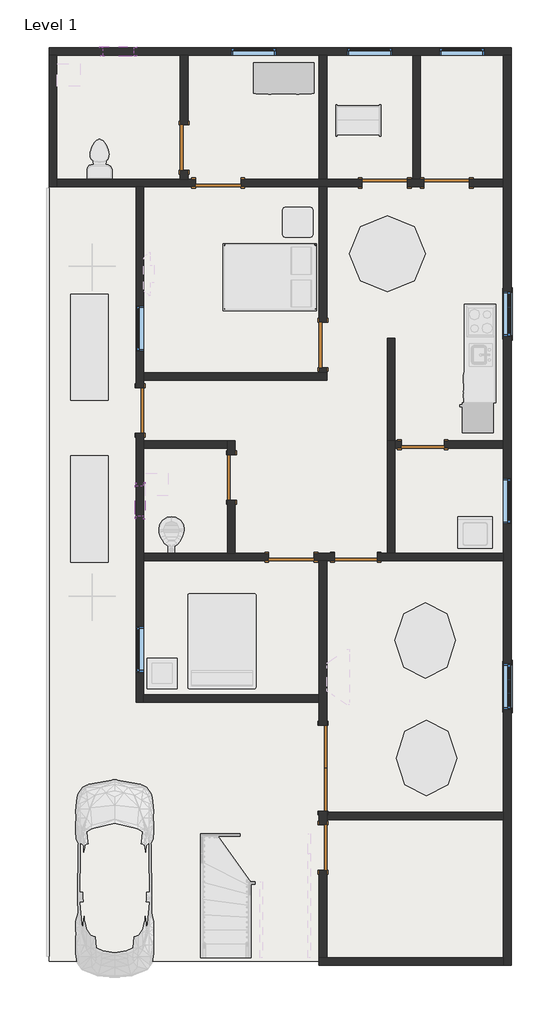
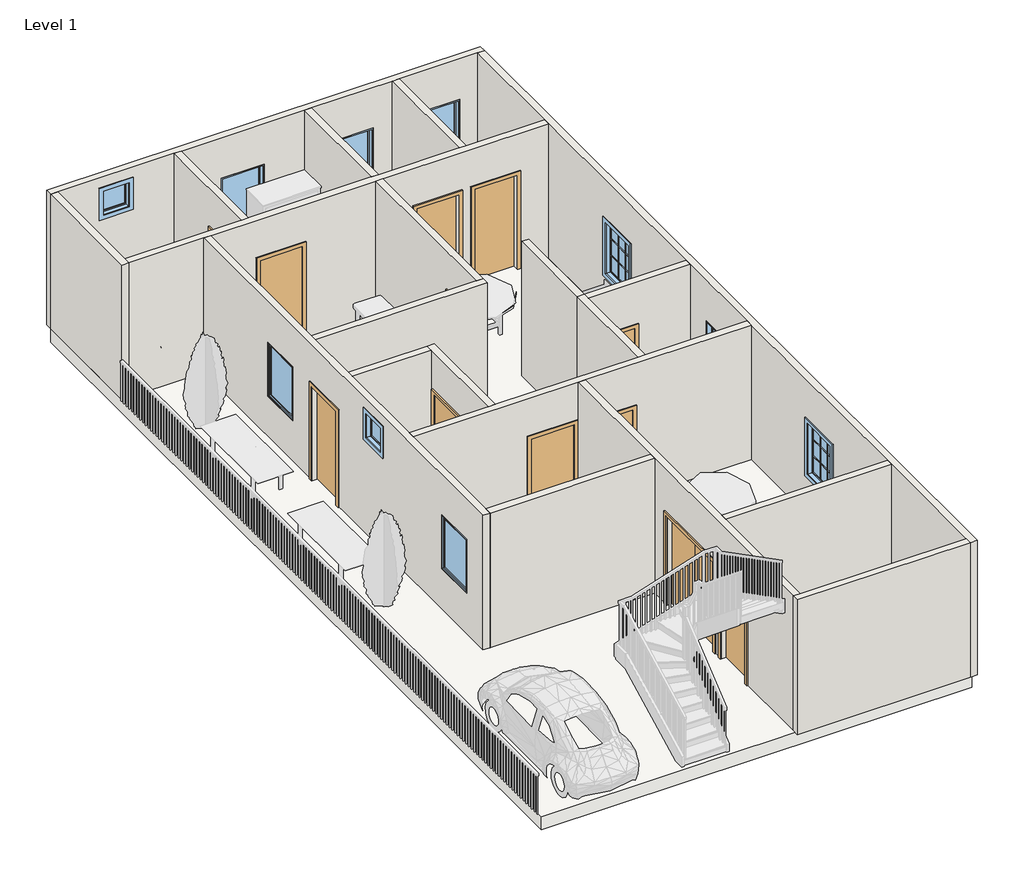
# One storey, part 1 of 4: 20 walls, 12 doors, 10 windows, 1 slab.
"""IFC4 building model written with IfcOpenShell, lengths in millimetres."""

from ifc_helpers import new_model, si_unit, frame, origin, origin_with_axes, place, context, project, spatial, polyline, outline, extrude, faceted_brep, transform, mapped, element, save
from components import door_74777eb6, door_56e8e0a9, door_686f89d2, door_16372e1c, window_5c190c7e, window_d657a5cb, window_3d781103

model = new_model("IFC4")

# Units and contexts
model_context = context("Model", 3, world=origin())
ifc_project = project(units=[si_unit("LENGTHUNIT", "METRE", prefix="MILLI")], contexts=[model_context])

# Site, building, storey
site = spatial("IfcSite", under=ifc_project)
building = spatial("IfcBuilding", under=site)
storey = spatial("IfcBuildingStorey", under=building, Name="Level 1", Elevation=0.0)

# Doors
placement = place(None, origin())
door_shape = door_74777eb6(model_context)
element("IfcDoor", 1, ObjectType="Door-Double-Flush_Panel : 68\" x 80\"", at=placement, inside=storey, context=model_context, shape_type="MappedRepresentation", body=[
    mapped(door_shape, transform((-6523.260887, -797.8089531, 0.0), x_axis=(0.0, -1.0, 0.0), y_axis=(1.0, 0.0, 0.0), z_axis=(0.0, 0.0, 1.0))),
])
door_2_shape = door_56e8e0a9(model_context)
element("IfcDoor", 2, ObjectType="Single-Flush : 34\" x 80\"", at=placement, inside=storey, context=model_context, shape_type="MappedRepresentation", body=[
    mapped(door_2_shape, transform((-5862.860887, 3443.9910469, 0.0), x_axis=(-1.0, 0.0, 0.0), y_axis=(0.0, -1.0, 0.0), z_axis=(0.0, 0.0, 1.0))),
])
element("IfcDoor", 3, ObjectType="Single-Flush : 34\" x 80\"", at=placement, inside=storey, context=model_context, shape_type="MappedRepresentation", body=[
    mapped(door_2_shape, transform((-4516.660887, 5704.5910469, 0.0), x_axis=(-1.0, 0.0, 0.0), y_axis=(0.0, -1.0, 0.0), z_axis=(0.0, 0.0, 1.0))),
])
door_3_shape = door_686f89d2(model_context)
element("IfcDoor", 4, ObjectType="Single-Flush : 36\" x 84\"", at=placement, inside=storey, context=model_context, shape_type="MappedRepresentation", body=[
    mapped(door_3_shape, transform((-9317.260887, 11673.5910469, 0.0), x_axis=(0.0, -1.0, 0.0), y_axis=(1.0, 0.0, 0.0), z_axis=(0.0, 0.0, 1.0))),
])
element("IfcDoor", 5, ObjectType="Single-Flush : 36\" x 84\"", at=placement, inside=storey, context=model_context, shape_type="MappedRepresentation", body=[
    mapped(door_3_shape, transform((-8631.460887, 10962.3910469, 0.0), x_axis=(1.0, 0.0, 0.0), y_axis=(0.0, 1.0, 0.0), z_axis=(0.0, 0.0, 1.0))),
])
element("IfcDoor", 6, ObjectType="Single-Flush : 36\" x 84\"", at=placement, inside=storey, context=model_context, shape_type="MappedRepresentation", body=[
    mapped(door_3_shape, transform((-4034.060887, 10962.3910469, 0.0), x_axis=(-1.0, 0.0, 0.0), y_axis=(0.0, -1.0, 0.0), z_axis=(0.0, 0.0, 1.0))),
])
element("IfcDoor", 7, ObjectType="Single-Flush : 36\" x 84\"", at=placement, inside=storey, context=model_context, shape_type="MappedRepresentation", body=[
    mapped(door_3_shape, transform((-6523.260887, 7711.1910469, 0.0), x_axis=(0.0, -1.0, 0.0), y_axis=(1.0, 0.0, 0.0), z_axis=(0.0, 0.0, 1.0))),
])
element("IfcDoor", 8, ObjectType="Single-Flush : 36\" x 84\"", at=placement, inside=storey, context=model_context, shape_type="MappedRepresentation", body=[
    mapped(door_3_shape, transform((-7158.260887, 3443.9910469, 0.0), x_axis=(1.0, 0.0, 0.0), y_axis=(0.0, 1.0, 0.0), z_axis=(0.0, 0.0, 1.0))),
])
element("IfcDoor", 9, ObjectType="Single-Flush : 36\" x 84\"", at=placement, inside=storey, context=model_context, shape_type="MappedRepresentation", body=[
    mapped(door_3_shape, transform((-6523.260887, -2398.0089531, 0.0), x_axis=(0.0, 1.0, 0.0), y_axis=(-1.0, 0.0, 0.0), z_axis=(0.0, 0.0, 1.0))),
])
door_4_shape = door_16372e1c(model_context)
element("IfcDoor", 10, ObjectType="Single-Flush : 36\" x 84\"", at=placement, inside=storey, context=model_context, shape_type="MappedRepresentation", body=[
    mapped(door_4_shape, transform((-5278.660887, 10962.3910469, 0.0), x_axis=(1.0, 0.0, 0.0), y_axis=(0.0, 1.0, 0.0), z_axis=(0.0, 0.0, 1.0))),
])
element("IfcDoor", 11, ObjectType="Single-Flush : 36\" x 84\"", at=placement, inside=storey, context=model_context, shape_type="MappedRepresentation", body=[
    mapped(door_4_shape, transform((-10206.260887, 6390.3910469, 0.0), x_axis=(0.0, -1.0, 0.0), y_axis=(1.0, 0.0, 0.0), z_axis=(0.0, 0.0, 1.0))),
])
element("IfcDoor", 12, ObjectType="Single-Flush : 36\" x 84\"", at=placement, inside=storey, context=model_context, shape_type="MappedRepresentation", body=[
    mapped(door_4_shape, transform((-8364.760887, 5044.1910469, 0.0), x_axis=(0.0, 1.0, 0.0), y_axis=(-1.0, 0.0, 0.0), z_axis=(0.0, 0.0, 1.0))),
])

# Slab
element("IfcSlab", 13, ObjectType="Generic - 12\"", at=placement, inside=storey, context=model_context, shape_type="SweptSolid", body=[
    extrude(outline(polyline([(-2814.860887, 13527.7910469), (-2814.860887, -4684.0089531), (-12035.060887, -4684.0089531), (-12035.060887, 13527.7910469), (-2814.860887, 13527.7910469)])), frame((0.0, 0.0, -304.8), z_axis=(0.0, 0.0, 1.0), x_axis=(1.0, 0.0, 0.0)), (0.0, 0.0, 1.0), 304.8),
])

# Walls
element("IfcWall", 14, ObjectType="Generic - 8\"", at=placement, inside=storey, context=model_context, shape_type="Brep", body=[
    faceted_brep([(-12035.060887, 13527.7910469, 0.0), (-11882.660887, 13527.7910469, 0.0), (-9393.460887, 13527.7910469, 0.0), (-9241.060887, 13527.7910469, 0.0), (-6599.460887, 13527.7910469, 0.0), (-6447.060887, 13527.7910469, 0.0), (-4719.860887, 13527.7910469, 0.0), (-4567.460887, 13527.7910469, 0.0), (-2891.060887, 13527.7910469, 0.0), (-2738.660887, 13527.7910469, 0.0), (-2738.660887, 13527.7910469, 3048.0), (-2891.060887, 13527.7910469, 3048.0), (-4567.460887, 13527.7910469, 3048.0), (-4719.860887, 13527.7910469, 3048.0), (-6447.060887, 13527.7910469, 3048.0), (-6599.460887, 13527.7910469, 3048.0), (-9241.060887, 13527.7910469, 3048.0), (-9393.460887, 13527.7910469, 3048.0), (-11882.660887, 13527.7910469, 3048.0), (-12035.060887, 13527.7910469, 3048.0), (-7463.060887, 13527.7910469, 2133.6), (-7463.060887, 13527.7910469, 914.4), (-8377.460887, 13527.7910469, 914.4), (-8377.460887, 13527.7910469, 2133.6), (-5126.260887, 13527.7910469, 2133.6), (-5126.260887, 13527.7910469, 914.4), (-6040.660887, 13527.7910469, 914.4), (-6040.660887, 13527.7910469, 2133.6), (-3272.060887, 13527.7910469, 2133.6), (-3272.060887, 13527.7910469, 914.4), (-4186.460887, 13527.7910469, 914.4), (-4186.460887, 13527.7910469, 2133.6), (-10333.260887, 13527.7910469, 2768.6), (-10333.260887, 13527.7910469, 2159.0), (-10942.860887, 13527.7910469, 2159.0), (-10942.860887, 13527.7910469, 2768.6), (-12035.060887, 13680.1910469, 0.0), (-12035.060887, 13680.1910469, 3048.0), (-2738.660887, 13680.1910469, 3048.0), (-2738.660887, 13680.1910469, 0.0), (-7463.060887, 13680.1910469, 2133.6), (-8377.460887, 13680.1910469, 2133.6), (-8377.460887, 13680.1910469, 914.4), (-7463.060887, 13680.1910469, 914.4), (-5126.260887, 13680.1910469, 2133.6), (-6040.660887, 13680.1910469, 2133.6), (-6040.660887, 13680.1910469, 914.4), (-5126.260887, 13680.1910469, 914.4), (-3272.060887, 13680.1910469, 2133.6), (-4186.460887, 13680.1910469, 2133.6), (-4186.460887, 13680.1910469, 914.4), (-3272.060887, 13680.1910469, 914.4), (-10333.260887, 13680.1910469, 2768.6), (-10942.860887, 13680.1910469, 2768.6), (-10942.860887, 13680.1910469, 2159.0), (-10333.260887, 13680.1910469, 2159.0)], [[[0, 1, 2, 3, 4, 5, 6, 7, 8, 9, 10, 11, 12, 13, 14, 15, 16, 17, 18, 19], [20, 21, 22, 23], [24, 25, 26, 27], [28, 29, 30, 31], [32, 33, 34, 35]], [[36, 37, 38, 39], [40, 41, 42, 43], [44, 45, 46, 47], [48, 49, 50, 51], [52, 53, 54, 55]], [[9, 8, 7, 6, 5, 4, 3, 2, 1, 0, 36, 39]], [[19, 18, 17, 16, 15, 14, 13, 12, 11, 10, 38, 37]], [[10, 9, 39, 38]], [[0, 19, 37, 36]], [[21, 20, 40, 43]], [[22, 21, 43, 42]], [[23, 22, 42, 41]], [[20, 23, 41, 40]], [[25, 24, 44, 47]], [[26, 25, 47, 46]], [[27, 26, 46, 45]], [[24, 27, 45, 44]], [[29, 28, 48, 51]], [[30, 29, 51, 50]], [[31, 30, 50, 49]], [[28, 31, 49, 48]], [[33, 32, 52, 55]], [[34, 33, 55, 54]], [[35, 34, 54, 53]], [[32, 35, 53, 52]]]),
])
element("IfcWall", 15, ObjectType="Generic - 8\"", at=placement, inside=storey, context=model_context, shape_type="Brep", body=[
    faceted_brep([(-2891.060887, 13527.7910469, 0.0), (-2891.060887, 11038.5910469, 0.0), (-2891.060887, 10886.1910469, 0.0), (-2891.060887, 5780.7910469, 0.0), (-2891.060887, 5628.3910469, 0.0), (-2891.060887, 3520.1910469, 0.0), (-2891.060887, 3367.7910469, 0.0), (-2891.060887, -1686.8089531, 0.0), (-2891.060887, -1839.2089531, 0.0), (-2891.060887, -4607.8089531, 0.0), (-2891.060887, -4760.2089531, 0.0), (-2891.060887, -4760.2089531, 3048.0), (-2891.060887, -4607.8089531, 3048.0), (-2891.060887, -1839.2089531, 3048.0), (-2891.060887, -1686.8089531, 3048.0), (-2891.060887, 3367.7910469, 3048.0), (-2891.060887, 3520.1910469, 3048.0), (-2891.060887, 5628.3910469, 3048.0), (-2891.060887, 5780.7910469, 3048.0), (-2891.060887, 10886.1910469, 3048.0), (-2891.060887, 11038.5910469, 3048.0), (-2891.060887, 13527.7910469, 3048.0), (-2891.060887, 4117.0910469, 2133.6), (-2891.060887, 4117.0910469, 914.4), (-2891.060887, 5031.4910469, 914.4), (-2891.060887, 5031.4910469, 2133.6), (-2891.060887, 383.2910469, 2133.6), (-2891.060887, 383.2910469, 914.4), (-2891.060887, 1297.6910469, 914.4), (-2891.060887, 1297.6910469, 2133.6), (-2891.060887, 7876.2910469, 2133.6), (-2891.060887, 7876.2910469, 914.4), (-2891.060887, 8790.6910469, 914.4), (-2891.060887, 8790.6910469, 2133.6), (-2738.660887, 13527.7910469, 0.0), (-2738.660887, 13527.7910469, 3048.0), (-2738.660887, -4760.2089531, 3048.0), (-2738.660887, -4760.2089531, 0.0), (-2738.660887, 4117.0910469, 2133.6), (-2738.660887, 5031.4910469, 2133.6), (-2738.660887, 5031.4910469, 914.4), (-2738.660887, 4117.0910469, 914.4), (-2738.660887, 383.2910469, 2133.6), (-2738.660887, 1297.6910469, 2133.6), (-2738.660887, 1297.6910469, 914.4), (-2738.660887, 383.2910469, 914.4), (-2738.660887, 7876.2910469, 2133.6), (-2738.660887, 8790.6910469, 2133.6), (-2738.660887, 8790.6910469, 914.4), (-2738.660887, 7876.2910469, 914.4)], [[[0, 1, 2, 3, 4, 5, 6, 7, 8, 9, 10, 11, 12, 13, 14, 15, 16, 17, 18, 19, 20, 21], [22, 23, 24, 25], [26, 27, 28, 29], [30, 31, 32, 33]], [[34, 35, 36, 37], [38, 39, 40, 41], [42, 43, 44, 45], [46, 47, 48, 49]], [[10, 9, 8, 7, 6, 5, 4, 3, 2, 1, 0, 34, 37]], [[21, 20, 19, 18, 17, 16, 15, 14, 13, 12, 11, 36, 35]], [[0, 21, 35, 34]], [[11, 10, 37, 36]], [[23, 22, 38, 41]], [[24, 23, 41, 40]], [[25, 24, 40, 39]], [[22, 25, 39, 38]], [[27, 26, 42, 45]], [[28, 27, 45, 44]], [[29, 28, 44, 43]], [[26, 29, 43, 42]], [[31, 30, 46, 49]], [[32, 31, 49, 48]], [[33, 32, 48, 47]], [[30, 33, 47, 46]]]),
])
element("IfcWall", 16, ObjectType="Generic - 8\"", at=placement, inside=storey, context=model_context, shape_type="Brep", body=[
    faceted_brep([(-2891.060887, -4607.8089531, 0.0), (-6447.060887, -4607.8089531, 0.0), (-6599.460887, -4607.8089531, 0.0), (-6599.460887, -4607.8089531, 3048.0), (-6447.060887, -4607.8089531, 3048.0), (-2891.060887, -4607.8089531, 3048.0), (-2891.060887, -4760.2089531, 0.0), (-2891.060887, -4760.2089531, 3048.0), (-6599.460887, -4760.2089531, 3048.0), (-6599.460887, -4760.2089531, 0.0)], [[[0, 1, 2, 3, 4, 5]], [[6, 7, 8, 9]], [[2, 1, 0, 6, 9]], [[5, 4, 3, 8, 7]], [[0, 5, 7, 6]], [[3, 2, 9, 8]]]),
])
element("IfcWall", 17, ObjectType="Generic - 8\"", at=placement, inside=storey, context=model_context, shape_type="Brep", body=[
    faceted_brep([(-4821.460887, 10886.1910469, 0.0), (-4491.260887, 10886.1910469, 0.0), (-4491.260887, 10886.1910469, 2133.6), (-3576.860887, 10886.1910469, 2133.6), (-3576.860887, 10886.1910469, 0.0), (-2891.060887, 10886.1910469, 0.0), (-2891.060887, 10886.1910469, 3048.0), (-6447.060887, 10886.1910469, 3048.0), (-6599.460887, 10886.1910469, 3048.0), (-10130.060887, 10886.1910469, 3048.0), (-10282.460887, 10886.1910469, 3048.0), (-11882.660887, 10886.1910469, 3048.0), (-11882.660887, 10886.1910469, 0.0), (-10282.460887, 10886.1910469, 0.0), (-10130.060887, 10886.1910469, 0.0), (-9088.660887, 10886.1910469, 0.0), (-9088.660887, 10886.1910469, 2133.6), (-8174.260887, 10886.1910469, 2133.6), (-8174.260887, 10886.1910469, 0.0), (-6599.460887, 10886.1910469, 0.0), (-6447.060887, 10886.1910469, 0.0), (-5735.860887, 10886.1910469, 0.0), (-5735.860887, 10886.1910469, 2133.6), (-4821.460887, 10886.1910469, 2133.6), (-4491.260887, 11038.5910469, 2133.6), (-4491.260887, 11038.5910469, 0.0), (-4567.460887, 11038.5910469, 0.0), (-4719.860887, 11038.5910469, 0.0), (-4821.460887, 11038.5910469, 0.0), (-4821.460887, 11038.5910469, 2133.6), (-5735.860887, 11038.5910469, 2133.6), (-5735.860887, 11038.5910469, 0.0), (-6447.060887, 11038.5910469, 0.0), (-6599.460887, 11038.5910469, 0.0), (-8174.260887, 11038.5910469, 0.0), (-8174.260887, 11038.5910469, 2133.6), (-9088.660887, 11038.5910469, 2133.6), (-9088.660887, 11038.5910469, 0.0), (-9241.060887, 11038.5910469, 0.0), (-9393.460887, 11038.5910469, 0.0), (-11882.660887, 11038.5910469, 0.0), (-11882.660887, 11038.5910469, 3048.0), (-9393.460887, 11038.5910469, 3048.0), (-9241.060887, 11038.5910469, 3048.0), (-6599.460887, 11038.5910469, 3048.0), (-6447.060887, 11038.5910469, 3048.0), (-4719.860887, 11038.5910469, 3048.0), (-4567.460887, 11038.5910469, 3048.0), (-2891.060887, 11038.5910469, 3048.0), (-2891.060887, 11038.5910469, 0.0), (-3576.860887, 11038.5910469, 0.0), (-3576.860887, 11038.5910469, 2133.6)], [[[0, 1, 2, 3, 4, 5, 6, 7, 8, 9, 10, 11, 12, 13, 14, 15, 16, 17, 18, 19, 20, 21, 22, 23]], [[24, 25, 26, 27, 28, 29, 30, 31, 32, 33, 34, 35, 36, 37, 38, 39, 40, 41, 42, 43, 44, 45, 46, 47, 48, 49, 50, 51]], [[15, 14, 13, 12, 40, 39, 38, 37]], [[21, 20, 19, 18, 34, 33, 32, 31]], [[50, 49, 5, 4]], [[28, 27, 26, 25, 1, 0]], [[11, 10, 9, 8, 7, 6, 48, 47, 46, 45, 44, 43, 42, 41]], [[6, 5, 49, 48]], [[12, 11, 41, 40]], [[35, 34, 18, 17]], [[36, 35, 17, 16]], [[37, 36, 16, 15]], [[29, 28, 0, 23]], [[30, 29, 23, 22]], [[31, 30, 22, 21]], [[2, 1, 25, 24]], [[3, 2, 24, 51]], [[4, 3, 51, 50]]]),
])
element("IfcWall", 18, ObjectType="Generic - 8\"", at=placement, inside=storey, context=model_context, shape_type="Brep", body=[
    faceted_brep([(-10282.460887, 5933.1910469, 2133.6), (-10282.460887, 5933.1910469, 0.0), (-10282.460887, 522.9910469, 0.0), (-10282.460887, 522.9910469, 3048.0), (-10282.460887, 10886.1910469, 3048.0), (-10282.460887, 10886.1910469, 0.0), (-10282.460887, 6847.5910469, 0.0), (-10282.460887, 6847.5910469, 2133.6), (-10282.460887, 8498.5910469, 2133.6), (-10282.460887, 7584.1910469, 2133.6), (-10282.460887, 7584.1910469, 914.4), (-10282.460887, 8498.5910469, 914.4), (-10282.460887, 2046.9910469, 2133.6), (-10282.460887, 1132.5910469, 2133.6), (-10282.460887, 1132.5910469, 914.4), (-10282.460887, 2046.9910469, 914.4), (-10282.460887, 4269.4910469, 2768.6), (-10282.460887, 4269.4910469, 2159.0), (-10282.460887, 4879.0910469, 2159.0), (-10282.460887, 4879.0910469, 2768.6), (-10130.060887, 522.9910469, 0.0), (-10130.060887, 675.3910469, 0.0), (-10130.060887, 3367.7910469, 0.0), (-10130.060887, 3520.1910469, 0.0), (-10130.060887, 5628.3910469, 0.0), (-10130.060887, 5780.7910469, 0.0), (-10130.060887, 5933.1910469, 0.0), (-10130.060887, 5933.1910469, 2133.6), (-10130.060887, 6847.5910469, 2133.6), (-10130.060887, 6847.5910469, 0.0), (-10130.060887, 6999.9910469, 0.0), (-10130.060887, 7152.3910469, 0.0), (-10130.060887, 10886.1910469, 0.0), (-10130.060887, 10886.1910469, 3048.0), (-10130.060887, 7152.3910469, 3048.0), (-10130.060887, 6999.9910469, 3048.0), (-10130.060887, 5780.7910469, 3048.0), (-10130.060887, 5628.3910469, 3048.0), (-10130.060887, 3520.1910469, 3048.0), (-10130.060887, 3367.7910469, 3048.0), (-10130.060887, 675.3910469, 3048.0), (-10130.060887, 522.9910469, 3048.0), (-10130.060887, 8498.5910469, 2133.6), (-10130.060887, 8498.5910469, 914.4), (-10130.060887, 7584.1910469, 914.4), (-10130.060887, 7584.1910469, 2133.6), (-10130.060887, 2046.9910469, 2133.6), (-10130.060887, 2046.9910469, 914.4), (-10130.060887, 1132.5910469, 914.4), (-10130.060887, 1132.5910469, 2133.6), (-10130.060887, 4269.4910469, 2768.6), (-10130.060887, 4879.0910469, 2768.6), (-10130.060887, 4879.0910469, 2159.0), (-10130.060887, 4269.4910469, 2159.0)], [[[0, 1, 2, 3, 4, 5, 6, 7], [8, 9, 10, 11], [12, 13, 14, 15], [16, 17, 18, 19]], [[20, 21, 22, 23, 24, 25, 26, 27, 28, 29, 30, 31, 32, 33, 34, 35, 36, 37, 38, 39, 40, 41], [42, 43, 44, 45], [46, 47, 48, 49], [50, 51, 52, 53]], [[6, 5, 32, 31, 30, 29]], [[2, 1, 26, 25, 24, 23, 22, 21, 20]], [[4, 3, 41, 40, 39, 38, 37, 36, 35, 34, 33]], [[5, 4, 33, 32]], [[3, 2, 20, 41]], [[27, 26, 1, 0]], [[28, 27, 0, 7]], [[29, 28, 7, 6]], [[43, 42, 8, 11]], [[44, 43, 11, 10]], [[45, 44, 10, 9]], [[42, 45, 9, 8]], [[47, 46, 12, 15]], [[48, 47, 15, 14]], [[49, 48, 14, 13]], [[46, 49, 13, 12]], [[17, 16, 50, 53]], [[18, 17, 53, 52]], [[19, 18, 52, 51]], [[16, 19, 51, 50]]]),
])
element("IfcWall", 19, ObjectType="Generic - 8\"", at=placement, inside=storey, context=model_context, shape_type="SweptSolid", body=[
    extrude(outline(polyline([(-6599.460887, 522.9910469), (-10130.060887, 522.9910469), (-10130.060887, 675.3910469), (-6599.460887, 675.3910469), (-6599.460887, 522.9910469)])), origin_with_axes(), (0.0, 0.0, 1.0), 3048.0),
])
element("IfcWall", 20, ObjectType="Generic - 8\"", at=placement, inside=storey, context=model_context, shape_type="Brep", body=[
    faceted_brep([(-6447.060887, 3367.7910469, 3048.0), (-6447.060887, -1686.8089531, 3048.0), (-6447.060887, -1839.2089531, 3048.0), (-6447.060887, -4607.8089531, 3048.0), (-6447.060887, -4607.8089531, 0.0), (-6447.060887, -2855.2089531, 0.0), (-6447.060887, -2855.2089531, 2133.6), (-6447.060887, -1940.8089531, 2133.6), (-6447.060887, -1940.8089531, 0.0), (-6447.060887, -1839.2089531, 0.0), (-6447.060887, -1686.8089531, 0.0), (-6447.060887, -1661.4089531, 0.0), (-6447.060887, -1661.4089531, 2032.0), (-6447.060887, 65.7910469, 2032.0), (-6447.060887, 65.7910469, 0.0), (-6447.060887, 3367.7910469, 0.0), (-6599.460887, -4607.8089531, 3048.0), (-6599.460887, 522.9910469, 3048.0), (-6599.460887, 675.3910469, 3048.0), (-6599.460887, 3367.7910469, 3048.0), (-6599.460887, 3367.7910469, 0.0), (-6599.460887, 675.3910469, 0.0), (-6599.460887, 522.9910469, 0.0), (-6599.460887, 65.7910469, 0.0), (-6599.460887, 65.7910469, 2032.0), (-6599.460887, -1661.4089531, 2032.0), (-6599.460887, -1661.4089531, 0.0), (-6599.460887, -1940.8089531, 0.0), (-6599.460887, -1940.8089531, 2133.6), (-6599.460887, -2855.2089531, 2133.6), (-6599.460887, -2855.2089531, 0.0), (-6599.460887, -4607.8089531, 0.0)], [[[0, 1, 2, 3, 4, 5, 6, 7, 8, 9, 10, 11, 12, 13, 14, 15]], [[16, 17, 18, 19, 20, 21, 22, 23, 24, 25, 26, 27, 28, 29, 30, 31]], [[4, 31, 30, 5]], [[20, 15, 14, 23, 22, 21]], [[8, 27, 26, 11, 10, 9]], [[3, 2, 1, 0, 19, 18, 17, 16]], [[0, 15, 20, 19]], [[4, 3, 16, 31]], [[28, 27, 8, 7]], [[29, 28, 7, 6]], [[30, 29, 6, 5]], [[25, 12, 11, 26]], [[12, 25, 24, 13]], [[13, 24, 23, 14]]]),
])
element("IfcWall", 21, ObjectType="Generic - 8\"", at=placement, inside=storey, context=model_context, shape_type="Brep", body=[
    faceted_brep([(-6294.660887, 3520.1910469, 2032.0), (-6294.660887, 3520.1910469, 0.0), (-6701.060887, 3520.1910469, 0.0), (-6701.060887, 3520.1910469, 2133.6), (-7615.460887, 3520.1910469, 2133.6), (-7615.460887, 3520.1910469, 0.0), (-8288.560887, 3520.1910469, 0.0), (-8440.960887, 3520.1910469, 0.0), (-10130.060887, 3520.1910469, 0.0), (-10130.060887, 3520.1910469, 3048.0), (-8440.960887, 3520.1910469, 3048.0), (-8288.560887, 3520.1910469, 3048.0), (-5227.860887, 3520.1910469, 3048.0), (-5075.460887, 3520.1910469, 3048.0), (-2891.060887, 3520.1910469, 3048.0), (-2891.060887, 3520.1910469, 0.0), (-5075.460887, 3520.1910469, 0.0), (-5227.860887, 3520.1910469, 0.0), (-5431.060887, 3520.1910469, 0.0), (-5431.060887, 3520.1910469, 2032.0), (-6701.060887, 3367.7910469, 0.0), (-6599.460887, 3367.7910469, 0.0), (-6447.060887, 3367.7910469, 0.0), (-6294.660887, 3367.7910469, 0.0), (-6294.660887, 3367.7910469, 2032.0), (-5431.060887, 3367.7910469, 2032.0), (-5431.060887, 3367.7910469, 0.0), (-2891.060887, 3367.7910469, 0.0), (-2891.060887, 3367.7910469, 3048.0), (-6447.060887, 3367.7910469, 3048.0), (-6599.460887, 3367.7910469, 3048.0), (-10130.060887, 3367.7910469, 3048.0), (-10130.060887, 3367.7910469, 0.0), (-7615.460887, 3367.7910469, 0.0), (-7615.460887, 3367.7910469, 2133.6), (-6701.060887, 3367.7910469, 2133.6)], [[[0, 1, 2, 3, 4, 5, 6, 7, 8, 9, 10, 11, 12, 13, 14, 15, 16, 17, 18, 19]], [[20, 21, 22, 23, 24, 25, 26, 27, 28, 29, 30, 31, 32, 33, 34, 35]], [[33, 32, 8, 7, 6, 5]], [[2, 1, 23, 22, 21, 20]], [[18, 17, 16, 15, 27, 26]], [[14, 13, 12, 11, 10, 9, 31, 30, 29, 28]], [[9, 8, 32, 31]], [[3, 2, 20, 35]], [[4, 3, 35, 34]], [[5, 4, 34, 33]], [[15, 14, 28, 27]], [[24, 23, 1, 0]], [[25, 24, 0, 19]], [[26, 25, 19, 18]]]),
])
element("IfcWall", 22, ObjectType="Generic - 8\"", at=placement, inside=storey, context=model_context, shape_type="Brep", body=[
    faceted_brep([(-8288.560887, 5501.3910469, 2133.6), (-8288.560887, 5501.3910469, 0.0), (-8288.560887, 5780.7910469, 0.0), (-8288.560887, 5780.7910469, 3048.0), (-8288.560887, 3520.1910469, 3048.0), (-8288.560887, 3520.1910469, 0.0), (-8288.560887, 4586.9910469, 0.0), (-8288.560887, 4586.9910469, 2133.6), (-8440.960887, 5780.7910469, 0.0), (-8440.960887, 5628.3910469, 0.0), (-8440.960887, 5501.3910469, 0.0), (-8440.960887, 5501.3910469, 2133.6), (-8440.960887, 4586.9910469, 2133.6), (-8440.960887, 4586.9910469, 0.0), (-8440.960887, 3520.1910469, 0.0), (-8440.960887, 3520.1910469, 3048.0), (-8440.960887, 5628.3910469, 3048.0), (-8440.960887, 5780.7910469, 3048.0)], [[[0, 1, 2, 3, 4, 5, 6, 7]], [[8, 9, 10, 11, 12, 13, 14, 15, 16, 17]], [[6, 5, 14, 13]], [[2, 1, 10, 9, 8]], [[4, 3, 17, 16, 15]], [[5, 4, 15, 14]], [[3, 2, 8, 17]], [[11, 10, 1, 0]], [[12, 11, 0, 7]], [[13, 12, 7, 6]]]),
])
element("IfcWall", 23, ObjectType="Generic - 8\"", at=placement, inside=storey, context=model_context, shape_type="SweptSolid", body=[
    extrude(outline(polyline([(-10130.060887, 5780.7910469), (-8440.960887, 5780.7910469), (-8440.960887, 5628.3910469), (-10130.060887, 5628.3910469), (-10130.060887, 5780.7910469)])), origin_with_axes(), (0.0, 0.0, 1.0), 3048.0),
])
element("IfcWall", 24, ObjectType="Generic - 8\"", at=placement, inside=storey, context=model_context, shape_type="Brep", body=[
    faceted_brep([(-10130.060887, 6999.9910469, 0.0), (-6447.060887, 6999.9910469, 0.0), (-6447.060887, 6999.9910469, 3048.0), (-10130.060887, 6999.9910469, 3048.0), (-10130.060887, 7152.3910469, 0.0), (-10130.060887, 7152.3910469, 3048.0), (-6599.460887, 7152.3910469, 3048.0), (-6447.060887, 7152.3910469, 3048.0), (-6447.060887, 7152.3910469, 0.0), (-6599.460887, 7152.3910469, 0.0)], [[[0, 1, 2, 3]], [[4, 5, 6, 7, 8, 9]], [[1, 0, 4, 9, 8]], [[3, 2, 7, 6, 5]], [[0, 3, 5, 4]], [[2, 1, 8, 7]]]),
])
element("IfcWall", 25, ObjectType="Generic - 8\"", at=placement, inside=storey, context=model_context, shape_type="SweptSolid", body=[
    extrude(outline(polyline([(7253.9910469, 2133.6), (7253.9910469, 0.0), (7152.3910469, 0.0), (7152.3910469, 3048.0), (10886.1910469, 3048.0), (10886.1910469, 0.0), (8168.3910469, 0.0), (8168.3910469, 2133.6), (7253.9910469, 2133.6)])), frame((-6599.460887, 0.0, 0.0), z_axis=(1.0, 0.0, 0.0), x_axis=(0.0, 1.0, 0.0)), (0.0, 0.0, 1.0), 152.4),
])
element("IfcWall", 26, ObjectType="Generic - 8\"", at=placement, inside=storey, context=model_context, shape_type="Brep", body=[
    faceted_brep([(-11882.660887, 10886.1910469, 0.0), (-11882.660887, 11038.5910469, 0.0), (-11882.660887, 13527.7910469, 0.0), (-11882.660887, 13527.7910469, 3048.0), (-11882.660887, 11038.5910469, 3048.0), (-11882.660887, 10886.1910469, 3048.0), (-12035.060887, 10886.1910469, 0.0), (-12035.060887, 10886.1910469, 3048.0), (-12035.060887, 13527.7910469, 3048.0), (-12035.060887, 13527.7910469, 0.0)], [[[0, 1, 2, 3, 4, 5]], [[6, 7, 8, 9]], [[2, 1, 0, 6, 9]], [[5, 4, 3, 8, 7]], [[3, 2, 9, 8]], [[0, 5, 7, 6]]]),
])
element("IfcWall", 27, ObjectType="Generic - 8\"", at=placement, inside=storey, context=model_context, shape_type="SweptSolid", body=[
    extrude(outline(polyline([(11216.3910469, 2133.6), (11216.3910469, 0.0), (11038.5910469, 0.0), (11038.5910469, 3048.0), (13527.7910469, 3048.0), (13527.7910469, 0.0), (12130.7910469, 0.0), (12130.7910469, 2133.6), (11216.3910469, 2133.6)])), frame((-9393.460887, 0.0, 0.0), z_axis=(1.0, 0.0, 0.0), x_axis=(0.0, 1.0, 0.0)), (0.0, 0.0, 1.0), 152.4),
])
element("IfcWall", 28, ObjectType="Generic - 8\"", at=placement, inside=storey, context=model_context, shape_type="SweptSolid", body=[
    extrude(outline(polyline([(-6599.460887, 11038.5910469), (-6599.460887, 13527.7910469), (-6447.060887, 13527.7910469), (-6447.060887, 11038.5910469), (-6599.460887, 11038.5910469)])), origin_with_axes(), (0.0, 0.0, 1.0), 3048.0),
])
element("IfcWall", 29, ObjectType="Generic - 8\"", at=placement, inside=storey, context=model_context, shape_type="SweptSolid", body=[
    extrude(outline(polyline([(-4719.860887, 11038.5910469), (-4719.860887, 13527.7910469), (-4567.460887, 13527.7910469), (-4567.460887, 11038.5910469), (-4719.860887, 11038.5910469)])), origin_with_axes(), (0.0, 0.0, 1.0), 3048.0),
])
element("IfcWall", 30, ObjectType="Generic - 8\"", at=placement, inside=storey, context=model_context, shape_type="SweptSolid", body=[
    extrude(outline(polyline([(-2891.060887, -1839.2089531), (-6447.060887, -1839.2089531), (-6447.060887, -1686.8089531), (-2891.060887, -1686.8089531), (-2891.060887, -1839.2089531)])), origin_with_axes(), (0.0, 0.0, 1.0), 3048.0),
])
element("IfcWall", 31, ObjectType="Generic - 8\"", at=placement, inside=storey, context=model_context, shape_type="Brep", body=[
    faceted_brep([(-5227.860887, 5780.7910469, 0.0), (-5227.860887, 3520.1910469, 0.0), (-5227.860887, 3520.1910469, 3048.0), (-5227.860887, 5780.7910469, 3048.0), (-5075.460887, 5780.7910469, 0.0), (-5075.460887, 5780.7910469, 3048.0), (-5075.460887, 5628.3910469, 3048.0), (-5075.460887, 3520.1910469, 3048.0), (-5075.460887, 3520.1910469, 0.0), (-5075.460887, 5628.3910469, 0.0)], [[[0, 1, 2, 3]], [[4, 5, 6, 7, 8, 9]], [[1, 0, 4, 9, 8]], [[3, 2, 7, 6, 5]], [[2, 1, 8, 7]], [[0, 3, 5, 4]]]),
])
element("IfcWall", 32, ObjectType="Generic - 8\"", at=placement, inside=storey, context=model_context, shape_type="SweptSolid", body=[
    extrude(outline(polyline([(0.0, -5075.460887), (0.0, -4948.460887), (2032.0, -4948.460887), (2032.0, -4084.860887), (0.0, -4084.860887), (0.0, -2891.060887), (3048.0, -2891.060887), (3048.0, -5075.460887), (0.0, -5075.460887)])), frame((0.0, 5628.3910469, 0.0), z_axis=(0.0, 1.0, 0.0), x_axis=(0.0, 0.0, 1.0)), (0.0, 0.0, 1.0), 152.4),
])
element("IfcWall", 33, ObjectType="Generic - 8\"", at=placement, inside=storey, context=model_context, shape_type="SweptSolid", body=[
    extrude(outline(polyline([(-5075.460887, 7838.1910469), (-5075.460887, 5780.7910469), (-5227.860887, 5780.7910469), (-5227.860887, 7838.1910469), (-5075.460887, 7838.1910469)])), origin_with_axes(), (0.0, 0.0, 1.0), 3048.0),
])

# Windows
window_shape = window_5c190c7e(model_context)
element("IfcWindow", 34, ObjectType="Casement 3x3 with Trim : 36\" x 48\"", at=placement, inside=storey, context=model_context, shape_type="MappedRepresentation", body=[
    mapped(window_shape, transform((-2814.860887, 840.4910469, 0.0), x_axis=(0.0, -1.0, 0.0), y_axis=(1.0, 0.0, 0.0), z_axis=(0.0, 0.0, 1.0))),
])
element("IfcWindow", 35, ObjectType="Casement 3x3 with Trim : 36\" x 48\"", at=placement, inside=storey, context=model_context, shape_type="MappedRepresentation", body=[
    mapped(window_shape, transform((-2814.860887, 8333.4910469, 0.0), x_axis=(0.0, -1.0, 0.0), y_axis=(1.0, 0.0, 0.0), z_axis=(0.0, 0.0, 1.0))),
])
window_2_shape = window_d657a5cb(model_context)
element("IfcWindow", 36, ObjectType="Fixed : 36\" x 48\"", at=placement, inside=storey, context=model_context, shape_type="MappedRepresentation", body=[
    mapped(window_2_shape, transform((-7882.160887, 13603.9910469, 0.0), x_axis=(1.0, 0.0, 0.0), y_axis=(0.0, 1.0, 0.0), z_axis=(0.0, 0.0, 1.0))),
])
element("IfcWindow", 37, ObjectType="Fixed : 36\" x 48\"", at=placement, inside=storey, context=model_context, shape_type="MappedRepresentation", body=[
    mapped(window_2_shape, transform((-5545.360887, 13603.9910469, 0.0), x_axis=(1.0, 0.0, 0.0), y_axis=(0.0, 1.0, 0.0), z_axis=(0.0, 0.0, 1.0))),
])
element("IfcWindow", 38, ObjectType="Fixed : 36\" x 48\"", at=placement, inside=storey, context=model_context, shape_type="MappedRepresentation", body=[
    mapped(window_2_shape, transform((-3691.160887, 13603.9910469, 0.0), x_axis=(1.0, 0.0, 0.0), y_axis=(0.0, 1.0, 0.0), z_axis=(0.0, 0.0, 1.0))),
])
element("IfcWindow", 39, ObjectType="Fixed : 36\" x 48\"", at=placement, inside=storey, context=model_context, shape_type="MappedRepresentation", body=[
    mapped(window_2_shape, transform((-10206.260887, 8079.4910469, 0.0), x_axis=(0.0, 1.0, 0.0), y_axis=(-1.0, 0.0, 0.0), z_axis=(0.0, 0.0, 1.0))),
])
element("IfcWindow", 40, ObjectType="Fixed : 36\" x 48\"", at=placement, inside=storey, context=model_context, shape_type="MappedRepresentation", body=[
    mapped(window_2_shape, transform((-10206.260887, 1627.8910469, 0.0), x_axis=(0.0, 1.0, 0.0), y_axis=(-1.0, 0.0, 0.0), z_axis=(0.0, 0.0, 1.0))),
])
element("IfcWindow", 41, ObjectType="Fixed : 36\" x 48\"", at=placement, inside=storey, context=model_context, shape_type="MappedRepresentation", body=[
    mapped(window_2_shape, transform((-2814.860887, 4536.1910469, 0.0), x_axis=(0.0, -1.0, 0.0), y_axis=(1.0, 0.0, 0.0), z_axis=(0.0, 0.0, 1.0))),
])
window_3_shape = window_3d781103(model_context)
element("IfcWindow", 42, ObjectType="Transom with Trim : 24\" x 24\"", at=placement, inside=storey, context=model_context, shape_type="MappedRepresentation", body=[
    mapped(window_3_shape, transform((-10599.960887, 13603.9910469, 0.0), x_axis=(1.0, 0.0, 0.0), y_axis=(0.0, 1.0, 0.0), z_axis=(0.0, 0.0, 1.0))),
])
element("IfcWindow", 43, ObjectType="Transom with Trim : 24\" x 24\"", at=placement, inside=storey, context=model_context, shape_type="MappedRepresentation", body=[
    mapped(window_3_shape, transform((-10206.260887, 4536.1910469, 0.0), x_axis=(0.0, -1.0, 0.0), y_axis=(1.0, 0.0, 0.0), z_axis=(0.0, 0.0, 1.0))),
])

save(model, "model.ifc")

# Revit data of these elements
# Type "Door-Double-Flush_Panel : 68\" x 80\""
#   Type Mark = "8"
#   Construction Type Id = "DOOR"
#   Assembly Code = "C1020"
#   Analytic Construction = "Wooden"
#   Thickness = 0' - 2"
#   Thermal Resistance (R) = 2.5876 (h·ft²·°F)/BTU
#   Swing Angle [instance default] = 90.00°
#   Panel Width = 2' - 10"
#   Heat Transfer Coefficient (U) = 0.3865 BTU/(h·ft²·°F)
#   Height = 6' - 8"
#   Trim Projection Ext = 0' - 1"
#   Trim Projection Int = 0' - 1"
#   Trim Width = 0' - 3"
#   Width = 5' - 8"
#   Define Thermal Properties by = 1
#   Panel Material = Wood - Birch - Solid Stained Light Low Gloss
#   Trim Material = Paint - Sienna
#   Visual Light Transmittance = 0
#   Solar Heat Gain Coefficient = 0
#   Function = (empty or 0)
#   Wall Closure = (empty or 0)
# Type "Single-Flush : 34\" x 80\""
#   Type Mark = "7"
#   Construction Type Id = "MDOOR"
#   Assembly Code = "C1020"
#   Analytic Construction = "Metal"
#   Thickness = 0' - 2"
#   Heat Transfer Coefficient (U) = 0.651978 BTU/(h·ft²·°F)
#   Height = 6' - 8"
#   Trim Projection Ext = 0' - 1"
#   Trim Projection Int = 0' - 1"
#   Trim Width = 0' - 3"
#   Width = 2' - 10"
#   Define Thermal Properties by = 1
#   Door Material = Door - Panel
#   Frame Material = Door - Frame
#   Visual Light Transmittance = 0
#   Solar Heat Gain Coefficient = 0
#   Function = (empty or 0)
#   Wall Closure = (empty or 0)
# Type "Single-Flush : 36\" x 84\""
#   Type Mark = "1"
#   Construction Type Id = "MDOOR"
#   Assembly Code = "C1020"
#   Analytic Construction = "Metal"
#   Thickness = 0' - 2"
#   Heat Transfer Coefficient (U) = 0.651978 BTU/(h·ft²·°F)
#   Height = 7' - 0"
#   Trim Projection Ext = 0' - 1"
#   Trim Projection Int = 0' - 1"
#   Trim Width = 0' - 3"
#   Width = 3' - 0"
#   Define Thermal Properties by = 1
#   Door Material = Door - Panel
#   Frame Material = Door - Frame
#   Visual Light Transmittance = 0
#   Solar Heat Gain Coefficient = 0
#   Function = (empty or 0)
#   Wall Closure = (empty or 0)
# Type "Generic - 12\""
#   Assembly Code = "B1010"
#   Function = 0
#   Layers, outside or top first: 1' - 0" no material (function 1)
# Type "Generic - 8\""
#   Assembly Code = "B2010"
#   Layers, outside or top first: 0' - 6" "Brick, Common" (function 1)
# Type "Casement 3x3 with Trim : 36\" x 48\""
#   Type Mark = "10"
#   Construction Type Id = "GSP4R"
#   Assembly Code = "B2020100"
#   Analytic Construction = "1/8 in Pilkington single glazing"
#   Visual Light Transmittance = 0.9
#   Solar Heat Gain Coefficient = 0.78
#   Heat Transfer Coefficient (U) = 0.6496 BTU/(h·ft²·°F)
#   Height = 4' - 0"
#   Default Sill Height = 3' - 0"
#   Trim Projection - Ext. = 0' - 0 1/2"
#   Trim Projection - Int. = 0' - 0 3/4"
#   Trim Width - Exterior = 0' - 3 1/2"
#   Trim Width - Interior = 0' - 3 1/2"
#   Width = 3' - 0"
#   Window Inset = 0' - 0 3/4"
#   Define Thermal Properties by = 1
#   Glass Pane Material = Glass
#   Sash Material = Sash
#   Trim Exterior Material = Trim
#   Trim Interior Material = Trim
#   Wall Closure = (empty or 0)
# Type "Fixed : 36\" x 48\""
#   Type Mark = "1"
#   Construction Type Id = "GSP4R"
#   Assembly Code = "B2020100"
#   Analytic Construction = "1/8 in Pilkington single glazing"
#   Visual Light Transmittance = 0.9
#   Solar Heat Gain Coefficient = 0.78
#   Heat Transfer Coefficient (U) = 0.6496 BTU/(h·ft²·°F)
#   Height = 4' - 0"
#   Default Sill Height = 3' - 0"
#   Width = 3' - 0"
#   Window Inset = 0' - 0 3/4"
#   Define Thermal Properties by = 1
#   Glass Pane Material = Glass
#   Sash Material = Sash
#   Wall Closure = (empty or 0)
# Type "Transom with Trim : 24\" x 24\""
#   Type Mark = "13"
#   Construction Type Id = "GSP4R"
#   Assembly Code = "B2020100"
#   Analytic Construction = "1/8 in Pilkington single glazing"
#   Visual Light Transmittance = 0.9
#   Solar Heat Gain Coefficient = 0.78
#   Heat Transfer Coefficient (U) = 0.6496 BTU/(h·ft²·°F)
#   Height = 2' - 0"
#   Default Sill Height = 7' - 1"
#   Trim Projection - Ext. = 0' - 0 1/2"
#   Trim Projection - Int. = 0' - 0 3/4"
#   Trim Width - Exterior = 0' - 3 1/2"
#   Trim Width - Interior = 0' - 3 1/2"
#   Width = 2' - 0"
#   Window Inset = 0' - 0 3/4"
#   Define Thermal Properties by = 1
#   Glass Pane Material = Glass
#   Sash Material = Sash
#   Trim Exterior Material = Trim
#   Trim Interior Material = Trim
#   Wall Closure = (empty or 0)
# Element 1 (IfcDoor, "Door-Double-Flush_Panel : 68\" x 80\"")
#   Swing Angle = 90.00°
#   Phase Created = New Construction
#   Materials on its faces: "Paint - Sienna", "Wood - Birch - Solid Stained Light Low Gloss"
# Elements 2, 3 (IfcDoor, "Single-Flush : 34\" x 80\"")
#   Phase Created = New Construction
#   Materials on its faces: "Door - Frame", "Door - Panel"
# Elements 4, 5, 6, 7, 8, 9, 10, 11, 12 (IfcDoor, "Single-Flush : 36\" x 84\"")
#   Phase Created = New Construction
#   Materials on its faces: "Door - Frame", "Door - Panel"
# Element 13 (IfcSlab, "Generic - 12\"")
#   Height Offset From Level = 0' - 0"
#   Phase Created = New Construction
#   Materials on its faces: "Default Floor"
# Elements 14, 15, 16, 17, 18, 19, 20, 21, 22, 23, 24, 25, 26, 27, 28, 29, 30, 31, 32, 33 (IfcWall, "Generic - 8\"")
#   Top Offset = 0' - 0"
#   Base Offset = 0' - 0"
#   Unconnected Height = 10' - 0"
#   wall height = 10' - 0"
#   Phase Created = New Construction
#   Base Constraint = Level 1
#   Materials on its faces: "Brick, Common"
# Element 34 (IfcWindow, "Casement 3x3 with Trim : 36\" x 48\"")
#   Mark = "7"
#   Phase Created = New Construction
#   Materials on its faces: "Sash", "Glass", "Trim"
# Element 35 (IfcWindow, "Casement 3x3 with Trim : 36\" x 48\"")
#   Mark = "8"
#   Phase Created = New Construction
#   Materials on its faces: "Sash", "Glass", "Trim"
# Element 36 (IfcWindow, "Fixed : 36\" x 48\"")
#   Mark = "1"
#   Phase Created = New Construction
#   Materials on its faces: "Sash", "Glass"
# Element 37 (IfcWindow, "Fixed : 36\" x 48\"")
#   Mark = "2"
#   Phase Created = New Construction
#   Materials on its faces: "Sash", "Glass"
# Element 38 (IfcWindow, "Fixed : 36\" x 48\"")
#   Mark = "3"
#   Phase Created = New Construction
#   Materials on its faces: "Sash", "Glass"
# Element 39 (IfcWindow, "Fixed : 36\" x 48\"")
#   Mark = "4"
#   Phase Created = New Construction
#   Materials on its faces: "Sash", "Glass"
# Element 40 (IfcWindow, "Fixed : 36\" x 48\"")
#   Mark = "5"
#   Phase Created = New Construction
#   Materials on its faces: "Sash", "Glass"
# Element 41 (IfcWindow, "Fixed : 36\" x 48\"")
#   Mark = "6"
#   Phase Created = New Construction
#   Materials on its faces: "Sash", "Glass"
# Element 42 (IfcWindow, "Transom with Trim : 24\" x 24\"")
#   Mark = "9"
#   Phase Created = New Construction
#   Materials on its faces: "Sash", "Trim", "Glass"
# Element 43 (IfcWindow, "Transom with Trim : 24\" x 24\"")
#   Mark = "10"
#   Phase Created = New Construction
#   Materials on its faces: "Sash", "Trim", "Glass"
# Materials
#   "Wood - Birch - Solid Stained Light Low Gloss": class "Wood", colour RGB 210 159 95, transparency 0, Cost = 0
#   "Paint - Sienna": colour RGB 118 70 51, transparency 0, Cost = 0
#   "Door - Panel": class "Wood", colour RGB 210 159 95, transparency 0
#   "Door - Frame": colour RGB 118 70 51, transparency 0
#   "Brick, Common": class "Masonry", colour RGB 170 98 104, transparency 0, Description = "Common brick", Cost = 0
#   "Glass": class "Glass", colour RGB 0 128 192, transparency 0.75, Description = "Soda Lime Glass", Cost = 0
#   "Sash": class "Wood", colour RGB 224 178 126, transparency 0
#   "Trim": class "Wood", colour RGB 224 178 126, transparency 0
#   "Default Floor": colour RGB 128 128 128, transparency 0
# Room at (-4074.232, 6695.836) mm, phase "New Construction", upper level "Level 1", upper offset 10' - 0", lower offset 0' - 0"
#   Number = "15"
#   Name = "KITCHEN"
# Room at (-10624.213, 12424.234) mm, phase "New Construction", upper level "Level 1", upper offset 10' - 0", lower offset 0' - 0"
#   Number = "1"
#   Name = "TOILET"
# Room at (-7853.182, 12424.234) mm, phase "New Construction", upper level "Level 1", upper offset 10' - 0", lower offset 0' - 0"
#   Number = "2"
# Room at (-5491.508, 12424.234) mm, phase "New Construction", upper level "Level 1", upper offset 10' - 0", lower offset 0' - 0"
#   Number = "3"
#   Name = "STORE"
# Room at (-3662.708, 12424.234) mm, phase "New Construction", upper level "Level 1", upper offset 10' - 0", lower offset 0' - 0"
#   Number = "4"
# Room at (-8795.413, 9243.847) mm, phase "New Construction", upper level "Level 1", upper offset 10' - 0", lower offset 0' - 0"
#   Number = "5"
#   Name = "BEDROOM"
# Room at (-4767.262, 9243.847) mm, phase "New Construction", upper level "Level 1", upper offset 10' - 0", lower offset 0' - 0"
#   Number = "6"
#   Name = "DINING"
# Room at (-6966.613, 5433.68) mm, phase "New Construction", upper level "Level 1", upper offset 10' - 0", lower offset 0' - 0"
#   Number = "7"
#   Name = "LOBBY"
# Room at (-4074.504, 4772.412) mm, phase "New Construction", upper level "Level 1", upper offset 10' - 0", lower offset 0' - 0"
#   Number = "8"
#   Name = "WASH AREA"
# Room at (-9333.164, 4772.412) mm, phase "New Construction", upper level "Level 1", upper offset 10' - 0", lower offset 0' - 0"
#   Number = "9"
#   Name = "TOILET"
# Room at (-8795.413, 2344.337) mm, phase "New Construction", upper level "Level 1", upper offset 10' - 0", lower offset 0' - 0"
#   Number = "10"
#   Name = "BED ROOM"
# Room at (-4498.718, 1681.792) mm, phase "New Construction", upper level "Level 1", upper offset 10' - 0", lower offset 0' - 0"
#   Number = "11"
#   Name = "LIVING ROOM"
# Room at (-4767.262, -2936.273) mm, phase "New Construction", upper level "Level 1", upper offset 10' - 0", lower offset 0' - 0"
#   Number = "12"
#   Name = "STORE"
# Room at (-9681.982, -1674.117) mm, phase "New Construction", upper level "Level 1", upper offset 10' - 0", lower offset 0' - 0"
#   Number = "13"
#   Name = "PARKING"
# Room at (-11161.964, 6695.836) mm, phase "New Construction", upper level "Level 1", upper offset 10' - 0", lower offset 0' - 0"
#   Number = "14"
#   Name = "BALCONY"
